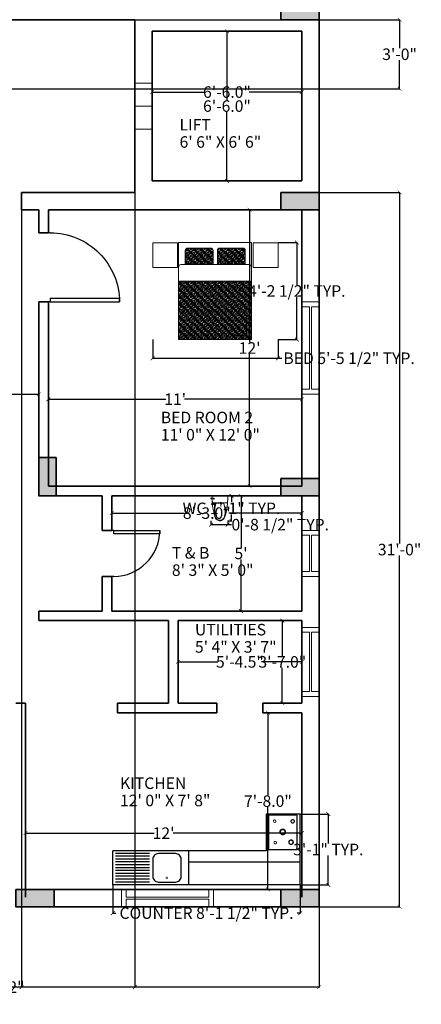
# Model space of a CAD drawing. Units: inches. Extents: x 560 to 1118, y 291 to 1226.
# Tile 2 of 4: x 886 to 1095, y 291 to 804. Entities that reach past the tile are written whole.
import ezdxf

# ---------------------------------------------------------------- set-up
doc = ezdxf.new("R2010")
doc.units = ezdxf.units.IN
doc.header["$MEASUREMENT"] = 0
for name, color, linetype, lineweight in [('A-ANNO-DIMS', 2, 'Continuous', 13), ('A-AREA-IDEN', 7, 'Continuous', 18), ('A-COLS', 7, 'Continuous', 35), ('A-FLOR-EVTR', 4, 'Continuous', 18), ('A-FLOR-FIXT', 9, 'Continuous', 18), ('DOORS', 4, 'Continuous', 25), ('FURNITURE', 8, 'Continuous', 18), ('WALL', 7, 'Continuous', 35), ('WINDOWS', 80, 'Continuous', 18)]:
    doc.layers.add(name, color=color, linetype=linetype, lineweight=lineweight)
doc.layers.add('DUVAR', color=7, linetype='Continuous')
doc.layers.add('TEFRIS', color=11, linetype='Continuous')
doc.styles.get("Standard").update_dxf_attribs({"font": 'arial.ttf'})
doc.dimstyles.get("Standard").update_dxf_attribs({"dimtxt": 6, "dimasz": 2, "dimexe": 0.18, "dimexo": 0.0625, "dimgap": 0.09, "dimtad": 0, "dimtih": 1, "dimtoh": 1, "dimdec": 1, "dimzin": 0, "dimdsep": 46, "dimlunit": 3, "dimtxsty": 'Standard', "dimblk": 'ARCHTICK', "dimcen": 0.09, "dimadec": 0, "dimazin": 0, "dimtfac": 1, "dimtdec": 1, "dimtofl": 0, "dimtmove": 0, "dimatfit": 3, "dimfxl": 1, "dimtolj": 1, "dimtzin": 0, "dimarcsym": 0})
pattern_1 = [(135, (-1377.70473, -125.71507), (-0.070710678, -0.070710678), []), (135, (-1377.68705, -125.69739), (-0.070710678, -0.070710678), []), (45, (-1377.70473, -125.71507), (-0.070710678, 0.070710678), [-0.025, 0.025]), (45, (-1377.72241, -125.69739), (-0.070710678, 0.070710678), [-0.025, 0.025]), (45, (-1377.74009, -125.67972), (-0.070710678, 0.070710678), [0.025, -0.025]), (45, (-1377.75776, -125.66204), (-0.070710678, 0.070710678), [0.025, -0.025]), (135, (-1377.66938, -125.67972), (-0.070710678, -0.070710678), [0.025, -0.025]), (135, (-1377.6517, -125.66204), (-0.070710678, -0.070710678), [0.025, -0.025])]

# ---------------------------------------------------------------- blocks, each defined once
blk = doc.blocks.new('*U3')
for p, q in [((0, 0), (0, -6)), ((36, 0), (36, -6))]:
    blk.add_line(p, q)
blk.add_lwpolyline([(0, 0), (0, 36), (1.75, 36), (1.75, 0)], close=True)
blk.add_arc((0, 0), 36, 0, 90)
blk = doc.blocks.new('*U4')
for p, q in [((0, 0), (0, -6)), ((24, 0), (24, -6))]:
    blk.add_line(p, q)
blk.add_lwpolyline([(0, 0), (0, 24), (1.75, 24), (1.75, 0)], close=True)
blk.add_arc((0, 0), 24, 0, 90)
blk = doc.blocks.new('_ArchTick')
at = {"color": 0, "linetype": 'ByBlock', "const_width": 0.15}
blk.add_lwpolyline([(-0.5, -0.5), (0.5, 0.5)], dxfattribs=at)
blk = doc.blocks.new('*D16')
at = {"layer": 'A-ANNO-DIMS', "color": 0, "lineweight": -2, "transparency": 16777216}
for p, q in [((994.18, 798), (994.18, 762.15)), ((994.24, 798), (994.36, 798)), ((994.18, 720), (994.18, 755.85)), ((994.24, 720), (994.36, 720))]:
    blk.add_line(p, q, dxfattribs=at)
at = {"layer": 'Defpoints', "color": 0, "transparency": 16777216}
for p in [(994.18, 798), (994.18, 720), (994.18, 720)]:
    blk.add_point(p, dxfattribs=at)
at = {"layer": 'A-ANNO-DIMS', "color": 0, "lineweight": -2, "transparency": 16777216, "xscale": 2, "yscale": 2, "zscale": 2}
for p, rotation in [((994.18, 798), 90), ((994.18, 720), 270)]:
    blk.add_blockref('_ArchTick', p, dxfattribs=dict(at, rotation=rotation))
at = {"layer": 'A-ANNO-DIMS', "color": 0, "transparency": 16777216, "insert": (994.18, 759), "char_height": 6, "attachment_point": 5}
blk.add_mtext('\\A1;6\'-6.0"', dxfattribs=at)
blk = doc.blocks.new('*D17')
at = {"layer": 'A-ANNO-DIMS', "color": 0, "lineweight": -2, "transparency": 16777216}
for p, q in [((955.18, 759.06), (955.18, 766.48)), ((955.18, 766.3), (982.6, 766.3)), ((1033.18, 766.3), (1005.76, 766.3)), ((1033.18, 759.06), (1033.18, 766.48))]:
    blk.add_line(p, q, dxfattribs=at)
at = {"layer": 'Defpoints', "color": 0, "transparency": 16777216}
for p in [(1033.18, 766.3), (955.18, 759), (1033.18, 759)]:
    blk.add_point(p, dxfattribs=at)
at = {"layer": 'A-ANNO-DIMS', "color": 0, "lineweight": -2, "transparency": 16777216, "xscale": 2, "yscale": 2, "zscale": 2, "rotation": 180}
blk.add_blockref('_ArchTick', (955.18, 766.3), dxfattribs=at)
at = {"layer": 'A-ANNO-DIMS', "color": 0, "lineweight": -2, "transparency": 16777216, "xscale": 2, "yscale": 2, "zscale": 2}
blk.add_blockref('_ArchTick', (1033.18, 766.3), dxfattribs=at)
at = {"layer": 'A-ANNO-DIMS', "color": 0, "transparency": 16777216, "insert": (994.18, 766.3), "char_height": 6, "attachment_point": 5}
blk.add_mtext('\\A1;6\'-6.0"', dxfattribs=at)
blk = doc.blocks.new('*D18')
at = {"layer": 'A-ANNO-DIMS', "color": 0, "lineweight": -2, "transparency": 16777216}
for p, q in [((901.18, 612.74), (901.18, 606.12)), ((1033.18, 611.44), (1033.18, 606.12)), ((901.18, 606.3), (962.28, 606.3)), ((1033.18, 606.3), (972.08, 606.3))]:
    blk.add_line(p, q, dxfattribs=at)
at = {"layer": 'Defpoints', "color": 0, "transparency": 16777216}
for p in [(901.18, 612.8), (1033.18, 611.5), (1033.18, 606.3)]:
    blk.add_point(p, dxfattribs=at)
at = {"layer": 'A-ANNO-DIMS', "color": 0, "lineweight": -2, "transparency": 16777216, "xscale": 2, "yscale": 2, "zscale": 2, "rotation": 180}
blk.add_blockref('_ArchTick', (901.18, 606.3), dxfattribs=at)
at = {"layer": 'A-ANNO-DIMS', "color": 0, "lineweight": -2, "transparency": 16777216, "xscale": 2, "yscale": 2, "zscale": 2}
blk.add_blockref('_ArchTick', (1033.18, 606.3), dxfattribs=at)
at = {"layer": 'A-ANNO-DIMS', "color": 0, "transparency": 16777216, "insert": (967.18, 606.3), "char_height": 6, "attachment_point": 5}
blk.add_mtext("\\A1;11'", dxfattribs=at)
blk = doc.blocks.new('*D19')
at = {"layer": 'A-ANNO-DIMS', "color": 0, "lineweight": -2, "transparency": 16777216}
for p, q in [((1006.94, 705), (1005.82, 705)), ((1006, 705), (1006, 636.1)), ((1006, 561), (1006, 629.9)), ((1006.94, 561), (1005.82, 561))]:
    blk.add_line(p, q, dxfattribs=at)
at = {"layer": 'Defpoints', "color": 0, "transparency": 16777216}
for p in [(1007, 705), (1006, 561), (1007, 561)]:
    blk.add_point(p, dxfattribs=at)
at = {"layer": 'A-ANNO-DIMS', "color": 0, "lineweight": -2, "transparency": 16777216, "xscale": 2, "yscale": 2, "zscale": 2}
for p, rotation in [((1006, 705), 90), ((1006, 561), 270)]:
    blk.add_blockref('_ArchTick', p, dxfattribs=dict(at, rotation=rotation))
at = {"layer": 'A-ANNO-DIMS', "color": 0, "transparency": 16777216, "insert": (1006, 633), "char_height": 6, "attachment_point": 5}
blk.add_mtext("\\A1;12'", dxfattribs=at)
blk = doc.blocks.new('*D20')
at = {"layer": 'A-ANNO-DIMS', "color": 0, "lineweight": -2, "transparency": 16777216}
for p, q in [((1001.94, 556), (1001.32, 556)), ((1001.5, 556), (1001.5, 529.14)), ((1001.5, 496), (1001.5, 522.86)), ((1001.94, 496), (1001.32, 496))]:
    blk.add_line(p, q, dxfattribs=at)
at = {"layer": 'Defpoints', "color": 0, "transparency": 16777216}
for p in [(1002, 556), (1001.5, 496), (1002, 496)]:
    blk.add_point(p, dxfattribs=at)
at = {"layer": 'A-ANNO-DIMS', "color": 0, "lineweight": -2, "transparency": 16777216, "xscale": 2, "yscale": 2, "zscale": 2}
for p, rotation in [((1001.5, 556), 90), ((1001.5, 496), 270)]:
    blk.add_blockref('_ArchTick', p, dxfattribs=dict(at, rotation=rotation))
at = {"layer": 'A-ANNO-DIMS', "color": 0, "transparency": 16777216, "insert": (1001.5, 526), "char_height": 6, "attachment_point": 5}
blk.add_mtext("\\A1;5'", dxfattribs=at)
blk = doc.blocks.new('*D21')
at = {"layer": 'A-ANNO-DIMS', "color": 0, "lineweight": -2, "transparency": 16777216}
for p, q in [((934.18, 547.06), (934.18, 547.18)), ((934.18, 547), (972.12, 547)), ((1033.18, 547), (995.24, 547)), ((1033.18, 543.86), (1033.18, 547.18))]:
    blk.add_line(p, q, dxfattribs=at)
at = {"layer": 'Defpoints', "color": 0, "transparency": 16777216}
for p in [(934.18, 547), (934.18, 547), (1033.18, 543.8)]:
    blk.add_point(p, dxfattribs=at)
at = {"layer": 'A-ANNO-DIMS', "color": 0, "lineweight": -2, "transparency": 16777216, "xscale": 2, "yscale": 2, "zscale": 2, "rotation": 180}
blk.add_blockref('_ArchTick', (934.18, 547), dxfattribs=at)
at = {"layer": 'A-ANNO-DIMS', "color": 0, "lineweight": -2, "transparency": 16777216, "xscale": 2, "yscale": 2, "zscale": 2}
blk.add_blockref('_ArchTick', (1033.18, 547), dxfattribs=at)
at = {"layer": 'A-ANNO-DIMS', "color": 0, "transparency": 16777216, "insert": (983.68, 547), "char_height": 6, "attachment_point": 5}
blk.add_mtext('\\A1;8\'-3.0"', dxfattribs=at)
blk = doc.blocks.new('*D22')
at = {"layer": 'A-ANNO-DIMS', "color": 0, "lineweight": -2, "transparency": 16777216}
for p, q in [((968.68, 469.5), (989.37, 469.5)), ((968.68, 469.44), (968.68, 469.32)), ((1033.18, 469.5), (1012.49, 469.5)), ((1033.18, 469.44), (1033.18, 469.32))]:
    blk.add_line(p, q, dxfattribs=at)
at = {"layer": 'Defpoints', "color": 0, "transparency": 16777216}
for p in [(968.68, 469.5), (1033.18, 469.5), (1033.18, 469.5)]:
    blk.add_point(p, dxfattribs=at)
at = {"layer": 'A-ANNO-DIMS', "color": 0, "lineweight": -2, "transparency": 16777216, "xscale": 2, "yscale": 2, "zscale": 2, "rotation": 180}
blk.add_blockref('_ArchTick', (968.68, 469.5), dxfattribs=at)
at = {"layer": 'A-ANNO-DIMS', "color": 0, "lineweight": -2, "transparency": 16777216, "xscale": 2, "yscale": 2, "zscale": 2}
blk.add_blockref('_ArchTick', (1033.18, 469.5), dxfattribs=at)
at = {"layer": 'A-ANNO-DIMS', "color": 0, "transparency": 16777216, "insert": (1000.93, 469.5), "char_height": 6, "attachment_point": 5}
blk.add_mtext('\\A1;5\'-4.5"', dxfattribs=at)
blk = doc.blocks.new('*D23')
at = {"layer": 'A-ANNO-DIMS', "color": 0, "lineweight": -2, "transparency": 16777216}
for p, q in [((1023, 491), (1023, 472.66)), ((1023.06, 491), (1023.18, 491)), ((1023, 448), (1023, 466.34)), ((1023.06, 448), (1023.18, 448))]:
    blk.add_line(p, q, dxfattribs=at)
at = {"layer": 'Defpoints', "color": 0, "transparency": 16777216}
for p in [(1023, 491), (1023, 448), (1023, 448)]:
    blk.add_point(p, dxfattribs=at)
at = {"layer": 'A-ANNO-DIMS', "color": 0, "lineweight": -2, "transparency": 16777216, "xscale": 2, "yscale": 2, "zscale": 2}
for p, rotation in [((1023, 491), 90), ((1023, 448), 270)]:
    blk.add_blockref('_ArchTick', p, dxfattribs=dict(at, rotation=rotation))
at = {"layer": 'A-ANNO-DIMS', "color": 0, "transparency": 16777216, "insert": (1023, 469.5), "char_height": 6, "attachment_point": 5}
blk.add_mtext('\\A1;3\'-7.0"', dxfattribs=at)
blk = doc.blocks.new('*D24')
at = {"layer": 'A-ANNO-DIMS', "color": 0, "lineweight": -2, "transparency": 16777216}
for p, q in [((889.18, 382.74), (889.18, 380.12)), ((889.18, 380.3), (956.28, 380.3)), ((1033.18, 380.3), (966.08, 380.3)), ((1033.18, 382.74), (1033.18, 380.12))]:
    blk.add_line(p, q, dxfattribs=at)
at = {"layer": 'Defpoints', "color": 0, "transparency": 16777216}
for p in [(889.18, 382.8), (1033.18, 382.8), (1033.18, 380.3)]:
    blk.add_point(p, dxfattribs=at)
at = {"layer": 'A-ANNO-DIMS', "color": 0, "lineweight": -2, "transparency": 16777216, "xscale": 2, "yscale": 2, "zscale": 2, "rotation": 180}
blk.add_blockref('_ArchTick', (889.18, 380.3), dxfattribs=at)
at = {"layer": 'A-ANNO-DIMS', "color": 0, "lineweight": -2, "transparency": 16777216, "xscale": 2, "yscale": 2, "zscale": 2}
blk.add_blockref('_ArchTick', (1033.18, 380.3), dxfattribs=at)
at = {"layer": 'A-ANNO-DIMS', "color": 0, "transparency": 16777216, "insert": (961.18, 380.3), "char_height": 6, "attachment_point": 5}
blk.add_mtext("\\A1;12'", dxfattribs=at)
blk = doc.blocks.new('*D25')
at = {"layer": 'A-ANNO-DIMS', "color": 0, "lineweight": -2, "transparency": 16777216}
for p, q in [((1018.44, 443), (1015.32, 443)), ((1015.5, 443), (1015.5, 400.15)), ((1015.5, 351), (1015.5, 393.85)), ((1018.44, 351), (1015.32, 351))]:
    blk.add_line(p, q, dxfattribs=at)
at = {"layer": 'Defpoints', "color": 0, "transparency": 16777216}
for p in [(1018.5, 443), (1015.5, 351), (1018.5, 351)]:
    blk.add_point(p, dxfattribs=at)
at = {"layer": 'A-ANNO-DIMS', "color": 0, "lineweight": -2, "transparency": 16777216, "xscale": 2, "yscale": 2, "zscale": 2}
for p, rotation in [((1015.5, 443), 90), ((1015.5, 351), 270)]:
    blk.add_blockref('_ArchTick', p, dxfattribs=dict(at, rotation=rotation))
at = {"layer": 'A-ANNO-DIMS', "color": 0, "transparency": 16777216, "insert": (1015.5, 397), "char_height": 6, "attachment_point": 5}
blk.add_mtext('\\A1;7\'-8.0"', dxfattribs=at)
blk = doc.blocks.new('*D43')
at = {"layer": 'A-ANNO-DIMS', "color": 0, "lineweight": -2, "transparency": 16777216}
for p, q in [((761.18, 606.56), (761.18, 608.98)), ((761.18, 608.8), (815.07, 608.8)), ((896.18, 608.8), (842.29, 608.8)), ((896.18, 606.56), (896.18, 608.98))]:
    blk.add_line(p, q, dxfattribs=at)
at = {"layer": 'Defpoints', "color": 0, "transparency": 16777216}
for p in [(761.18, 606.5), (896.18, 608.8), (896.18, 606.5)]:
    blk.add_point(p, dxfattribs=at)
at = {"layer": 'A-ANNO-DIMS', "color": 0, "lineweight": -2, "transparency": 16777216, "xscale": 2, "yscale": 2, "zscale": 2, "rotation": 180}
blk.add_blockref('_ArchTick', (761.18, 608.8), dxfattribs=at)
at = {"layer": 'A-ANNO-DIMS', "color": 0, "lineweight": -2, "transparency": 16777216, "xscale": 2, "yscale": 2, "zscale": 2}
blk.add_blockref('_ArchTick', (896.18, 608.8), dxfattribs=at)
at = {"layer": 'A-ANNO-DIMS', "color": 0, "transparency": 16777216, "insert": (828.68, 608.8), "char_height": 6, "attachment_point": 5}
blk.add_mtext('\\A1;11\'-3.0"', dxfattribs=at)
blk = doc.blocks.new('MAT-P10')
h = blk.add_hatch()
h.set_pattern_fill('BOX', color=256, scale=0.1, angle=45, style=0)
h.set_pattern_definition(pattern_1)
h.paths.add_polyline_path([(-0.157, 1.46), (0.417, 1.46), (0.417, 1.751, 0.414214), (0.367, 1.801), (-0.107, 1.801, 0.414214), (-0.157, 1.751)])
h.paths.add_polyline_path([(0.505, 1.46), (1.079, 1.46), (1.079, 1.751, 0.414214), (1.029, 1.801), (0.555, 1.801, 0.414214), (0.505, 1.751)])
h = blk.add_hatch()
h.set_pattern_fill('BOX', color=256, scale=0.1, angle=45, style=0)
h.set_pattern_definition(pattern_1)
edge = h.paths.add_edge_path()
edge.add_line((1.205, -0.085), (1.205, 1.062))
edge.add_ellipse((1.161, 1.063), major_axis=(0, 0.0568), ratio=0.776379, start_angle=270, end_angle=360)
edge.add_line((1.161, 1.119), (-0.251, 1.12))
edge.add_ellipse((-0.251, 1.063), major_axis=(0, 0.0568), ratio=0.776379, start_angle=0, end_angle=88.1396)
edge.add_line((-0.295, 1.064), (-0.295, -0.085))
edge.add_line((-0.295, -0.085), (1.205, -0.085))
for p, q in [((-0.251, 1.46), (1.161, 1.46)), ((-0.251, 1.12), (1.161, 1.119)), ((1.102, 0.406), (1.102, 0.057)), ((1.058, 0), (0.775, 0))]:
    blk.add_line(p, q)
for points in [[(-0.83, 1.909), (-0.319, 1.909), (-0.319, 1.398), (-0.83, 1.398)], [(1.205, -0.085), (-0.295, -0.085), (-0.295, 1.915), (1.205, 1.915)], [(1.244, 1.909), (1.755, 1.909), (1.755, 1.398), (1.244, 1.398)]]:
    blk.add_lwpolyline(points, close=True)
for points in [[(0.417, 1.46), (0.417, 1.751, 0.414214), (0.367, 1.801), (-0.107, 1.801, 0.414214), (-0.157, 1.751), (-0.157, 1.46)], [(1.079, 1.46), (1.079, 1.751, 0.414214), (1.029, 1.801), (0.555, 1.801, 0.414214), (0.505, 1.751), (0.505, 1.46)], [(1.012, 1.644), (1.012, 1.571, -0.414214), (0.962, 1.521), (0.753, 1.521)], [(0.37, 1.624), (0.37, 1.571, -0.414214), (0.32, 1.521), (0.111, 1.521)]]:
    blk.add_lwpolyline(points, format="xyb")
at = {"extrusion": (0, 0, -1)}
for centre, start_param, end_param in [((-0.251, 1.404), 4.712389, 6.283185), ((1.161, 1.404), 0, 1.570796), ((-0.251, 1.063), 4.712389, 6.283185), ((1.161, 1.063), 0, 1.570796), ((1.058, 0.057), 1.570796, 3.141593), ((1.058, 0.057), 1.570796, 3.141593)]:
    blk.add_ellipse(centre, major_axis=(0, 0.0568), ratio=0.776379, start_param=start_param, end_param=end_param, dxfattribs=at)
blk = doc.blocks.new('A$C3F871443')
at = {"layer": 'DUVAR'}
blk.add_line((3, 0), (3.3, 0), dxfattribs=at)
at = {"layer": 'TEFRIS'}
for p, q in [((0, 0), (0, -1.25)), ((0, 0), (3.3, 0)), ((1.97, -0.6), (1.97, 0)), ((3.3, 0), (3.3, -0.6)), ((3.253, -0.055), (2.653, -0.055)), ((2.653, -0.105), (3.253, -0.105)), ((2.653, -0.155), (3.253, -0.155)), ((2.653, -0.205), (3.253, -0.205)), ((2.653, -0.255), (3.253, -0.255)), ((2.653, -0.305), (3.253, -0.305)), ((0, -0.4), (1.97, -0.4)), ((2.653, -0.355), (3.253, -0.355)), ((2.653, -0.405), (3.253, -0.405)), ((2.653, -0.455), (3.253, -0.455)), ((2.653, -0.505), (3.253, -0.505)), ((0.6, -0.6), (3.3, -0.6)), ((0.6, -1.25), (0.6, -0.6)), ((2.653, -0.555), (3.253, -0.555)), ((0, -1.25), (0.6, -1.25))]:
    blk.add_line(p, q, dxfattribs=at)
blk.add_lwpolyline([(2.597, -0.452), (2.597, -0.152, 0.414214), (2.497, -0.052), (2.197, -0.052, 0.414214), (2.097, -0.152), (2.097, -0.452, 0.414214), (2.197, -0.552), (2.497, -0.552, 0.414214)], format="xyb", close=True, dxfattribs=at)
for points, const_width in [([(2.349, -0.141, 1), (2.349, -0.111, 1)], 0.01), ([(0.161, -0.791, 1), (0.161, -0.716, 1)], 0.025), ([(0.439, -0.768, 1), (0.439, -0.723, 1)], 0.015), ([(0.308, -0.98, 1), (0.308, -0.89, 1)], 0.03), ([(0.133, -1.151, 1), (0.133, -1.091, 1)], 0.02), ([(0.452, -1.147, 1), (0.452, -1.102, 1)], 0.015)]:
    blk.add_lwpolyline(points, format="xyb", close=True, dxfattribs=dict(at, const_width=const_width))
blk.add_lwpolyline([(0.556, -1.228), (0.556, -0.628), (0.056, -0.628), (0.056, -1.228)], close=True, dxfattribs=at)
blk = doc.blocks.new('toilet-7')
at = {"color": 0, "linetype": 'ByBlock'}
for p, q in [((-0.246, -0.087), (-0.246, -0.107)), ((-0.246, -0.087), (-0.226, -0.087)), ((-0.246, -0.107), (-0.226, -0.107)), ((-0.121, -0.237), (-0.228, -0.237)), ((-0.228, -0.237), (-0.228, -0.26)), ((-0.176, -0.26), (-0.228, -0.26)), ((-0.226, -0.085), (-0.226, -0.11)), ((-0.226, -0.085), (-0.216, -0.085)), ((-0.226, -0.11), (-0.215, -0.11)), ((0.21, -0.02), (-0.21, -0.02)), ((0.199, -0.212), (-0.199, -0.212)), ((-0.18, -0.237), (-0.18, -0.212)), ((-0.176, -0.26), (-0.138, -0.245)), ((-0.138, -0.245), (-0.138, -0.237)), ((-0.121, -0.237), (-0.121, -0.212)), ((-0.102, -0.221), (0.102, -0.221)), ((0.199, -0.212), (0.21, -0.164)), ((0.215, -0.068), (0.21, -0.02)), ((0.21, -0.164), (0.215, -0.117)), ((0.215, -0.117), (0.215, -0.068))]:
    blk.add_line(p, q, dxfattribs=at)
blk.add_circle((-0.17, -0.097), 0.0125, dxfattribs=at)
for centre, radius, start, end in [((0.224, -0.092), 0.44, 170.5377, 187.7399), ((1.517, -0.087), 1.732, 181.2224, 184.9822), ((0.224, -0.092), 0.44, 187.7399, 195.822), ((1.517, -0.087), 1.732, 185.7323, 197.2477), ((0.426, -0.441), 0.572, 157.3737, 194.7786), ((-0.426, -0.441), 0.572, 345.2214, 22.6263), ((-1.517, -0.087), 1.732, 342.7523, 358.7776), ((0.012, -0.554), 0.155, 197.2477, 249.5476), ((0.022, -0.548), 0.155, 194.7786, 226.8543), ((0, -0.571), 0.122, 226.8543, 313.1457), ((0, -0.585), 0.122, 249.5476, 290.4524), ((-0.012, -0.554), 0.155, 290.4524, 342.7523), ((-0.022, -0.548), 0.155, 313.1457, 345.2214)]:
    blk.add_arc(centre, radius, start, end, dxfattribs=at)
blk = doc.blocks.new('WIN-48IN')
for p, q in [((0, 9), (48, 9)), ((0, 0), (0, 9)), ((2.5, 5), (2.5, 9)), ((45.5, 9), (45.5, 5)), ((48, 9), (48, 0)), ((48, 0), (0, 0)), ((2.5, 5), (45.5, 5)), ((2.5, 0), (2.5, 4)), ((2.5, 4), (45.5, 4)), ((45.5, 4), (45.5, 0))]:
    blk.add_line(p, q)
blk = doc.blocks.new('WIN-36IN')
for p, q in [((0, 0), (0, 36)), ((0, 36), (9, 36)), ((9, 36), (9, 0)), ((0, 33.5), (4, 33.5)), ((4, 33.5), (4, 2.5)), ((5, 33.5), (9, 33.5)), ((5, 33.5), (5, 2.5)), ((4, 2.5), (0, 2.5)), ((9, 0), (0, 0)), ((9, 2.5), (5, 2.5))]:
    blk.add_line(p, q)
blk = doc.blocks.new('WIN-24IN')
for p, q in [((0, 0), (0, 24)), ((0, 24), (9, 24)), ((0, 21.5), (4, 21.5)), ((4, 21.5), (4, 2.5)), ((5, 21.5), (9, 21.5)), ((5, 21.5), (5, 2.5)), ((9, 24), (9, 0)), ((4, 2.5), (0, 2.5)), ((9, 0), (0, 0)), ((9, 2.5), (5, 2.5))]:
    blk.add_line(p, q)
blk = doc.blocks.new('COL-RECT-9X20-NOM')
h = blk.add_hatch(color=256)
h.dxf.hatch_style = 1
h.paths.add_polyline_path([(19.98, 0), (19.98, 9), (0, 9), (0, 0)])
blk.add_lwpolyline([(0, 9), (0, 0), (19.98, 0), (19.98, 9)], close=True)
blk = doc.blocks.new('*D61')
at = {"layer": 'A-ANNO-DIMS', "color": 0, "lineweight": -2, "transparency": 16777216}
for p, q in [((955.5, 637.39), (955.5, 627.48)), ((1020.77, 637.39), (1020.77, 627.48)), ((955.5, 627.66), (1020.77, 627.66)), ((1020.77, 627.66), (1022.77, 627.66))]:
    blk.add_line(p, q, dxfattribs=at)
at = {"layer": 'Defpoints', "color": 0, "transparency": 16777216}
for p in [(955.5, 637.45), (1020.77, 637.45), (1020.77, 627.66)]:
    blk.add_point(p, dxfattribs=at)
at = {"layer": 'A-ANNO-DIMS', "color": 0, "lineweight": -2, "transparency": 16777216, "xscale": 2, "yscale": 2, "zscale": 2, "rotation": 180}
blk.add_blockref('_ArchTick', (955.5, 627.66), dxfattribs=at)
at = {"layer": 'A-ANNO-DIMS', "color": 0, "lineweight": -2, "transparency": 16777216, "xscale": 2, "yscale": 2, "zscale": 2}
blk.add_blockref('_ArchTick', (1020.77, 627.66), dxfattribs=at)
at = {"layer": 'A-ANNO-DIMS', "color": 0, "transparency": 16777216, "insert": (1057.79, 627.66), "char_height": 6, "attachment_point": 5}
blk.add_mtext('\\A1;BED 5\'-5 1/2" TYP.', dxfattribs=at)
blk = doc.blocks.new('*D62')
at = {"layer": 'A-ANNO-DIMS', "color": 0, "lineweight": -2, "transparency": 16777216}
for p, q in [((1020.84, 687.95), (1030.75, 687.95)), ((1030.57, 687.95), (1030.57, 665.89)), ((1030.57, 637.45), (1030.57, 659.51)), ((1020.84, 637.45), (1030.75, 637.45))]:
    blk.add_line(p, q, dxfattribs=at)
at = {"layer": 'Defpoints', "color": 0, "transparency": 16777216}
for p in [(1020.77, 687.95), (1030.57, 687.95), (1020.77, 637.45)]:
    blk.add_point(p, dxfattribs=at)
at = {"layer": 'A-ANNO-DIMS', "color": 0, "lineweight": -2, "transparency": 16777216, "xscale": 2, "yscale": 2, "zscale": 2}
for p, rotation in [((1030.57, 687.95), 90), ((1030.57, 637.45), 270)]:
    blk.add_blockref('_ArchTick', p, dxfattribs=dict(at, rotation=rotation))
at = {"layer": 'A-ANNO-DIMS', "color": 0, "transparency": 16777216, "insert": (1030.57, 662.7), "char_height": 6, "attachment_point": 5}
blk.add_mtext('\\A1;4\'-2 1/2" TYP.', dxfattribs=at)
blk = doc.blocks.new('*D65')
at = {"layer": 'A-ANNO-DIMS', "color": 0, "lineweight": -2, "transparency": 16777216}
for p, q in [((994.63, 556), (996.7, 556)), ((996.52, 556), (996.52, 552.67)), ((996.52, 542.95), (996.52, 546.28)), ((994.63, 542.95), (996.7, 542.95))]:
    blk.add_line(p, q, dxfattribs=at)
at = {"layer": 'Defpoints', "color": 0, "transparency": 16777216}
for p in [(994.57, 556), (996.52, 556), (994.57, 542.95)]:
    blk.add_point(p, dxfattribs=at)
at = {"layer": 'A-ANNO-DIMS', "color": 0, "lineweight": -2, "transparency": 16777216, "xscale": 2, "yscale": 2, "zscale": 2}
for p, rotation in [((996.52, 556), 90), ((996.52, 542.95), 270)]:
    blk.add_blockref('_ArchTick', p, dxfattribs=dict(at, rotation=rotation))
at = {"layer": 'A-ANNO-DIMS', "color": 0, "transparency": 16777216, "insert": (996.52, 549.48), "char_height": 6, "attachment_point": 5}
blk.add_mtext('\\A1;WC 1\'-1" TYP.', dxfattribs=at)
blk = doc.blocks.new('*D66')
at = {"layer": 'A-ANNO-DIMS', "color": 0, "lineweight": -2, "transparency": 16777216}
for p, q in [((985.86, 542.89), (985.86, 540.81)), ((985.86, 540.99), (994.57, 540.99)), ((994.57, 542.89), (994.57, 540.81)), ((994.57, 540.99), (996.57, 540.99))]:
    blk.add_line(p, q, dxfattribs=at)
at = {"layer": 'Defpoints', "color": 0, "transparency": 16777216}
for p in [(985.86, 542.95), (994.57, 542.95), (994.57, 540.99)]:
    blk.add_point(p, dxfattribs=at)
at = {"layer": 'A-ANNO-DIMS', "color": 0, "lineweight": -2, "transparency": 16777216, "xscale": 2, "yscale": 2, "zscale": 2, "rotation": 180}
blk.add_blockref('_ArchTick', (985.86, 540.99), dxfattribs=at)
at = {"layer": 'A-ANNO-DIMS', "color": 0, "lineweight": -2, "transparency": 16777216, "xscale": 2, "yscale": 2, "zscale": 2}
blk.add_blockref('_ArchTick', (994.57, 540.99), dxfattribs=at)
at = {"layer": 'A-ANNO-DIMS', "color": 0, "transparency": 16777216, "insert": (1021.93, 540.99), "char_height": 6, "attachment_point": 5}
blk.add_mtext('\\A1;0\'-8 1/2" TYP.', dxfattribs=at)
blk = doc.blocks.new('*D69')
at = {"layer": 'A-ANNO-DIMS', "color": 0, "lineweight": -2, "transparency": 16777216}
for p, q in [((934.74, 353.24), (934.74, 338.48)), ((1032.33, 353.24), (1032.33, 338.48)), ((934.74, 338.66), (936.32, 338.66)), ((1032.33, 338.66), (1030.76, 338.66))]:
    blk.add_line(p, q, dxfattribs=at)
at = {"layer": 'Defpoints', "color": 0, "transparency": 16777216}
for p in [(934.74, 353.3), (1032.33, 353.3), (934.74, 338.66)]:
    blk.add_point(p, dxfattribs=at)
at = {"layer": 'A-ANNO-DIMS', "color": 0, "lineweight": -2, "transparency": 16777216, "xscale": 2, "yscale": 2, "zscale": 2, "rotation": 180}
blk.add_blockref('_ArchTick', (934.74, 338.66), dxfattribs=at)
at = {"layer": 'A-ANNO-DIMS', "color": 0, "lineweight": -2, "transparency": 16777216, "xscale": 2, "yscale": 2, "zscale": 2}
blk.add_blockref('_ArchTick', (1032.33, 338.66), dxfattribs=at)
at = {"layer": 'A-ANNO-DIMS', "color": 0, "transparency": 16777216, "insert": (983.54, 338.66), "char_height": 6, "attachment_point": 5}
blk.add_mtext('\\A1;COUNTER 8\'-1 1/2" TYP.', dxfattribs=at)
blk = doc.blocks.new('*D70')
at = {"layer": 'A-ANNO-DIMS', "color": 0, "lineweight": -2, "transparency": 16777216}
for p, q in [((1032.39, 390.26), (1047.15, 390.26)), ((1046.97, 390.26), (1046.97, 374.94)), ((1046.97, 353.3), (1046.97, 368.63)), ((1032.39, 353.3), (1047.15, 353.3))]:
    blk.add_line(p, q, dxfattribs=at)
at = {"layer": 'Defpoints', "color": 0, "transparency": 16777216}
for p in [(1032.33, 390.26), (1032.33, 353.3), (1046.97, 353.3)]:
    blk.add_point(p, dxfattribs=at)
at = {"layer": 'A-ANNO-DIMS', "color": 0, "lineweight": -2, "transparency": 16777216, "xscale": 2, "yscale": 2, "zscale": 2}
for p, rotation in [((1046.97, 390.26), 90), ((1046.97, 353.3), 270)]:
    blk.add_blockref('_ArchTick', p, dxfattribs=dict(at, rotation=rotation))
at = {"layer": 'A-ANNO-DIMS', "color": 0, "transparency": 16777216, "insert": (1046.97, 371.78), "char_height": 6, "attachment_point": 5}
blk.add_mtext('\\A1;3\'-1" TYP.', dxfattribs=at)
blk = doc.blocks.new('*D71')
at = {"layer": 'A-ANNO-DIMS', "color": 0, "lineweight": -2, "transparency": 16777216}
for p, q in [((615.18, 341.94), (615.18, 299.92)), ((1042.18, 341.94), (1042.18, 299.92)), ((615.18, 300.1), (818.29, 300.1)), ((1042.18, 300.1), (839.07, 300.1))]:
    blk.add_line(p, q, dxfattribs=at)
at = {"layer": 'Defpoints', "color": 0, "transparency": 16777216}
for p in [(615.18, 342), (1042.18, 342), (1042.18, 300.1)]:
    blk.add_point(p, dxfattribs=at)
at = {"layer": 'A-ANNO-DIMS', "color": 0, "lineweight": -2, "transparency": 16777216, "xscale": 2, "yscale": 2, "zscale": 2, "rotation": 180}
blk.add_blockref('_ArchTick', (615.18, 300.1), dxfattribs=at)
at = {"layer": 'A-ANNO-DIMS', "color": 0, "lineweight": -2, "transparency": 16777216, "xscale": 2, "yscale": 2, "zscale": 2}
blk.add_blockref('_ArchTick', (1042.18, 300.1), dxfattribs=at)
at = {"layer": 'A-ANNO-DIMS', "color": 0, "transparency": 16777216, "insert": (828.68, 300.1), "char_height": 6, "attachment_point": 5}
blk.add_mtext('\\A1;35\'-7"', dxfattribs=at)
blk = doc.blocks.new('*D76')
at = {"layer": 'A-ANNO-DIMS', "color": 0, "lineweight": -2, "transparency": 16777216}
for p, q in [((803.64, 713.94), (803.64, 299.92)), ((887.18, 713.94), (887.18, 299.92)), ((803.64, 300.1), (828.01, 300.1)), ((887.18, 300.1), (862.81, 300.1))]:
    blk.add_line(p, q, dxfattribs=at)
at = {"layer": 'Defpoints', "color": 0, "transparency": 16777216}
for p in [(803.64, 714), (887.18, 714), (887.18, 300.1)]:
    blk.add_point(p, dxfattribs=at)
at = {"layer": 'A-ANNO-DIMS', "color": 0, "lineweight": -2, "transparency": 16777216, "xscale": 2, "yscale": 2, "zscale": 2, "rotation": 180}
blk.add_blockref('_ArchTick', (803.64, 300.1), dxfattribs=at)
at = {"layer": 'A-ANNO-DIMS', "color": 0, "lineweight": -2, "transparency": 16777216, "xscale": 2, "yscale": 2, "zscale": 2}
blk.add_blockref('_ArchTick', (887.18, 300.1), dxfattribs=at)
at = {"layer": 'A-ANNO-DIMS', "color": 0, "transparency": 16777216, "insert": (845.41, 300.1), "char_height": 6, "attachment_point": 5}
blk.add_mtext('\\A1;6\'-11 1/2"', dxfattribs=at)
blk = doc.blocks.new('*D77')
at = {"layer": 'A-ANNO-DIMS', "color": 0, "lineweight": -2, "transparency": 16777216}
for p, q in [((946.18, 770.94), (946.18, 299.92)), ((794.64, 767.94), (794.64, 299.92)), ((794.64, 300.1), (853.3, 300.1)), ((946.18, 300.1), (887.51, 300.1))]:
    blk.add_line(p, q, dxfattribs=at)
at = {"layer": 'Defpoints', "color": 0, "transparency": 16777216}
for p in [(946.18, 771), (794.64, 768), (946.18, 300.1)]:
    blk.add_point(p, dxfattribs=at)
at = {"layer": 'A-ANNO-DIMS', "color": 0, "lineweight": -2, "transparency": 16777216, "xscale": 2, "yscale": 2, "zscale": 2, "rotation": 180}
blk.add_blockref('_ArchTick', (794.64, 300.1), dxfattribs=at)
at = {"layer": 'A-ANNO-DIMS', "color": 0, "lineweight": -2, "transparency": 16777216, "xscale": 2, "yscale": 2, "zscale": 2}
blk.add_blockref('_ArchTick', (946.18, 300.1), dxfattribs=at)
at = {"layer": 'A-ANNO-DIMS', "color": 0, "transparency": 16777216, "insert": (870.41, 300.1), "char_height": 6, "attachment_point": 5}
blk.add_mtext('\\A1;12\'-7 1/2"', dxfattribs=at)
blk = doc.blocks.new('*D78')
at = {"layer": 'A-ANNO-DIMS', "color": 0, "lineweight": -2, "transparency": 16777216}
for p, q in [((794.7, 804), (1084.26, 804)), ((1084.08, 804), (1084.08, 789.16)), ((1084.08, 768), (1084.08, 782.84)), ((794.7, 768), (1084.26, 768))]:
    blk.add_line(p, q, dxfattribs=at)
at = {"layer": 'Defpoints', "color": 0, "transparency": 16777216}
for p in [(794.64, 804), (1084.08, 804), (794.64, 768)]:
    blk.add_point(p, dxfattribs=at)
at = {"layer": 'A-ANNO-DIMS', "color": 0, "lineweight": -2, "transparency": 16777216, "xscale": 2, "yscale": 2, "zscale": 2}
for p, rotation in [((1084.08, 804), 90), ((1084.08, 768), 270)]:
    blk.add_blockref('_ArchTick', p, dxfattribs=dict(at, rotation=rotation))
at = {"layer": 'A-ANNO-DIMS', "color": 0, "transparency": 16777216, "insert": (1084.08, 786), "char_height": 6, "attachment_point": 5}
blk.add_mtext('\\A1;3\'-0"', dxfattribs=at)
blk = doc.blocks.new('*D79')
at = {"layer": 'A-ANNO-DIMS', "color": 0, "lineweight": -2, "transparency": 16777216}
for p, q in [((1042.24, 714), (1084.26, 714)), ((1084.08, 714), (1084.08, 531.16)), ((1084.08, 342), (1084.08, 524.84)), ((1042.24, 342), (1084.26, 342))]:
    blk.add_line(p, q, dxfattribs=at)
at = {"layer": 'Defpoints', "color": 0, "transparency": 16777216}
for p in [(1042.18, 714), (1084.08, 714), (1042.18, 342)]:
    blk.add_point(p, dxfattribs=at)
at = {"layer": 'A-ANNO-DIMS', "color": 0, "lineweight": -2, "transparency": 16777216, "xscale": 2, "yscale": 2, "zscale": 2}
for p, rotation in [((1084.08, 714), 90), ((1084.08, 342), 270)]:
    blk.add_blockref('_ArchTick', p, dxfattribs=dict(at, rotation=rotation))
at = {"layer": 'A-ANNO-DIMS', "color": 0, "transparency": 16777216, "insert": (1084.08, 528), "char_height": 6, "attachment_point": 5}
blk.add_mtext('\\A1;31\'-0"', dxfattribs=at)

msp = doc.modelspace()

# ---------------------------------------------------------------- linework, layer by layer
at = {"layer": 'A-FLOR-EVTR'}
for p, q in [((955.18, 771), (946.18, 771)), ((955.18, 759), (946.18, 759)), ((955.18, 747), (946.18, 747))]:
    msp.add_line(p, q, dxfattribs=at)
at = {"layer": 'WALL'}
for p, q in [((1042.18, 1180), (1042.18, 342)), ((946.18, 804), (878.18, 804)), ((946.18, 804), (946.18, 714)), ((955.18, 798), (955.18, 720)), ((1033.18, 798), (955.18, 798)), ((1033.18, 798), (1033.18, 720)), ((1033.18, 720), (955.18, 720)), ((946.18, 714), (887.18, 714)), ((887.18, 705), (887.18, 714)), ((896.18, 705), (887.18, 705)), ((896.18, 705), (896.18, 693)), ((1033.18, 705), (901.18, 705)), ((901.18, 705), (901.18, 693)), ((1033.18, 705), (1033.18, 561)), ((896.18, 693), (901.18, 693)), ((896.18, 657), (901.18, 657)), ((896.18, 657), (896.18, 556)), ((901.18, 657), (901.18, 561)), ((1033.18, 561), (901.18, 561)), ((929.18, 556), (896.18, 556)), ((929.18, 556), (929.18, 538)), ((1033.18, 556), (934.18, 556)), ((934.18, 556), (934.18, 538)), ((1033.18, 556), (1033.18, 496)), ((934.18, 538), (929.18, 538)), ((934.18, 514), (929.18, 514)), ((929.18, 514), (929.18, 496)), ((934.18, 514), (934.18, 496)), ((896.18, 496), (896.18, 491)), ((929.18, 496), (896.18, 496)), ((896.18, 496), (929.18, 496)), ((1033.18, 496), (934.18, 496)), ((934.18, 496), (1033.18, 496)), ((896.18, 491), (963.68, 491)), ((963.68, 491), (901.18, 491)), ((963.68, 491), (963.68, 448)), ((1033.18, 491), (968.68, 491)), ((968.68, 491), (968.68, 448)), ((968.68, 491), (1033.18, 491)), ((1033.18, 491), (1033.18, 448)), ((884.18, 448), (889.18, 448)), ((889.18, 443), (889.18, 448)), ((937.18, 443), (937.18, 448)), ((937.18, 448), (963.68, 448)), ((968.68, 448), (988.93, 448)), ((988.93, 448), (988.93, 443)), ((1012.93, 448), (1012.93, 443)), ((1012.93, 448), (1033.18, 448)), ((889.18, 443), (889.18, 347)), ((937.18, 443), (988.93, 443)), ((1012.93, 443), (1033.18, 443)), ((1033.18, 443), (1033.18, 347)), ((884.18, 351), (1042.18, 351)), ((884.18, 342), (1042.18, 342))]:
    msp.add_line(p, q, dxfattribs=at)

# ---------------------------------------------------------------- block references
at = {"layer": 'A-COLS'}
for p in [(1022.2, 804), (1022.2, 705), (1022.2, 556), (884.18, 342), (1022.2, 342)]:
    msp.add_blockref('COL-RECT-9X20-NOM', p, dxfattribs=at)
at = {"layer": 'A-COLS', "rotation": 270.0000000000005}
msp.add_blockref('COL-RECT-9X20-NOM', (896.18, 575.98), dxfattribs=at)
at = {"layer": 'A-FLOR-FIXT', "xscale": 18.9039470471375, "yscale": 18.9039470471375, "zscale": 18.9039470471375}
msp.add_blockref('toilet-7', (990.5, 556.38), dxfattribs=at)
at = {"layer": 'A-FLOR-FIXT', "xscale": 29.57142857142857, "yscale": 29.57142857142857, "zscale": 29.57142857142857, "rotation": 180}
msp.add_blockref('A$C3F871443', (1032.33, 353.3), dxfattribs=at)
at = {"layer": 'DOORS', "xscale": -1, "rotation": 270.0000000000002}
msp.add_blockref('*U3', (902.18, 657), dxfattribs=at)
at = {"layer": 'DOORS', "rotation": 270}
msp.add_blockref('*U4', (935.18, 538), dxfattribs=at)
at = {"layer": 'FURNITURE', "xscale": 25.25, "yscale": 25.25, "zscale": 25.25}
msp.add_blockref('MAT-P10', (976.46, 639.59), dxfattribs=at)
at = {"layer": 'WINDOWS'}
for name, p, rotation in [('WIN-48IN', (1033.18, 657), 270), ('WIN-24IN', (1042.18, 538), 180), ('WIN-36IN', (1042.18, 487.5), 180)]:
    msp.add_blockref(name, p, dxfattribs=dict(at, rotation=rotation))
msp.add_blockref('WIN-48IN', (939.18, 342), dxfattribs=at)

# ---------------------------------------------------------------- texts
at = {"layer": 'A-AREA-IDEN'}
for s, p in [('LIFT', (969.5, 746.3)), ('6\' 6" X 6\' 6"', (969.5, 737.3)), ('BED ROOM 2', (959.73, 593.8)), ('11\' 0" X 12\' 0"', (959.73, 584.8)), ('T & B', (965.5, 523.3)), ('8\' 3" X 5\' 0"', (965.5, 514.3)), ('UTILITIES', (977.5, 483.3)), ('5\' 4" X 3\' 7"', (977.5, 474.3)), ('KITCHEN', (938.5, 403.3)), ('12\' 0" X 7\' 8"', (938.5, 394.3))]:
    msp.add_text(s, height=6, dxfattribs=at).set_placement(p)

# ---------------------------------------------------------------- dimensions: what is measured, and where the dimension line sits
at = {"layer": 'A-ANNO-DIMS'}
for base, p1, p2, override, picture, middle in [((1084.08, 804), (794.64, 768), (794.64, 804), {"dimdec": 1, "dimlfac": 1, "dimrnd": 0, "dimzin": 1, "dimdsep": 46, "dimlunit": 4, "dimfrac": 2}, '*D78', (1084.08, 786)), ((994.18, 720), (994.18, 798), (994.18, 720), {"dimclrd": 0, "dimclre": 0, "dimclrt": 0}, '*D16', (994.18, 759)), ((1084.08, 714), (1042.18, 342), (1042.18, 714), {"dimdec": 1, "dimlfac": 1, "dimrnd": 0, "dimzin": 1, "dimdsep": 46, "dimlunit": 4, "dimfrac": 2}, '*D79', (1084.08, 528)), ((1006, 561), (1007, 705), (1007, 561), {"dimclrd": 0, "dimclre": 0, "dimclrt": 0}, '*D19', (1006, 633)), ((1001.5, 496), (1002, 556), (1002, 496), {"dimclrd": 0, "dimclre": 0, "dimclrt": 0}, '*D20', (1001.5, 526)), ((1023, 448), (1023, 491), (1023, 448), {"dimclrd": 0, "dimclre": 0, "dimclrt": 0}, '*D23', (1023, 469.5)), ((1015.5, 351), (1018.5, 443), (1018.5, 351), {"dimclrd": 0, "dimclre": 0, "dimclrt": 0}, '*D25', (1015.5, 397))]:
    dim = msp.add_linear_dim(base=base, p1=p1, p2=p2, angle=90, dimstyle='Standard', override=override, dxfattribs=at)
    dim.commit()
    dim.dimension.update_dxf_attribs({"geometry": picture, "text_midpoint": middle})
for base, p1, p2, override, picture, middle in [((946.18, 300.1), (794.64, 768), (946.18, 771), {"dimdec": 1, "dimlfac": 1, "dimrnd": 0, "dimzin": 1, "dimdsep": 46, "dimlunit": 4, "dimfrac": 2}, '*D77', (870.41, 300.1)), ((1033.18, 766.3), (955.18, 759), (1033.18, 759), {"dimclrd": 0, "dimclre": 0, "dimclrt": 0}, '*D17', (994.18, 766.3)), ((887.18, 300.1), (803.64, 714), (887.18, 714), {"dimdec": 1, "dimlfac": 1, "dimrnd": 0, "dimzin": 1, "dimdsep": 46, "dimlunit": 4, "dimfrac": 2}, '*D76', (845.41, 300.1)), ((896.18, 608.8), (761.18, 606.5), (896.18, 606.5), {"dimclrd": 0, "dimclre": 0, "dimclrt": 0}, '*D43', (828.68, 608.8)), ((1033.18, 606.3), (901.18, 612.8), (1033.18, 611.5), {"dimclrd": 0, "dimclre": 0, "dimclrt": 0}, '*D18', (967.18, 606.3)), ((934.18, 547), (1033.18, 543.8), (934.18, 547), {"dimclrd": 0, "dimclre": 0, "dimclrt": 0}, '*D21', (983.68, 547)), ((1033.18, 469.5), (968.68, 469.5), (1033.18, 469.5), {"dimclrd": 0, "dimclre": 0, "dimclrt": 0}, '*D22', (1000.93, 469.5)), ((1033.18, 380.3), (889.18, 382.8), (1033.18, 382.8), {"dimclrd": 0, "dimclre": 0, "dimclrt": 0}, '*D24', (961.18, 380.3)), ((1042.18, 300.1), (615.18, 342), (1042.18, 342), {"dimdec": 1, "dimlfac": 1, "dimrnd": 0, "dimzin": 1, "dimdsep": 46, "dimlunit": 4, "dimfrac": 2}, '*D71', (828.68, 300.1))]:
    dim = msp.add_linear_dim(base=base, p1=p1, p2=p2, dimstyle='Standard', override=override, dxfattribs=at)
    dim.commit()
    dim.dimension.update_dxf_attribs({"geometry": picture, "text_midpoint": middle})
for base, p1, p2, angle, text, picture, middle in [((1030.57, 687.95), (1020.77, 637.45), (1020.77, 687.95), 90, '<> TYP.', '*D62', (1030.57, 662.7)), ((996.523, 556), (994.5657, 542.9514), (994.5657, 556), 90, 'WC <> TYP.', '*D65', (996.523, 549.4757)), ((1046.97, 353.3), (1032.33, 390.26), (1032.33, 353.3), 270, '<> TYP.', '*D70', (1046.97, 371.78)), ((934.74, 338.66), (1032.33, 353.3), (934.74, 353.3), 180, 'COUNTER <> TYP.', '*D69', (983.54, 338.66))]:
    dim = msp.add_linear_dim(base=base, p1=p1, p2=p2, angle=angle, text=text, dimstyle='Standard', override={"dimdec": 1, "dimlfac": 1, "dimrnd": 0, "dimzin": 1, "dimdsep": 46, "dimlunit": 4, "dimfrac": 2}, dxfattribs=at)
    dim.commit()
    dim.dimension.update_dxf_attribs({"geometry": picture, "text_midpoint": middle})
for base, p1, p2, text, picture, middle in [((1020.77, 627.66), (955.5, 637.45), (1020.77, 637.45), 'BED <> TYP.', '*D61', (1057.79, 627.66)), ((994.57, 540.99), (985.86, 542.95), (994.57, 542.95), '<> TYP.', '*D66', (1021.93, 540.99))]:
    dim = msp.add_linear_dim(base=base, p1=p1, p2=p2, text=text, dimstyle='Standard', override={"dimdec": 1, "dimlfac": 1, "dimrnd": 0, "dimzin": 1, "dimdsep": 46, "dimlunit": 4, "dimfrac": 2}, dxfattribs=at)
    dim.commit()
    dim.dimension.update_dxf_attribs({"geometry": picture, "text_midpoint": middle})

doc.saveas('drawing.dxf')
